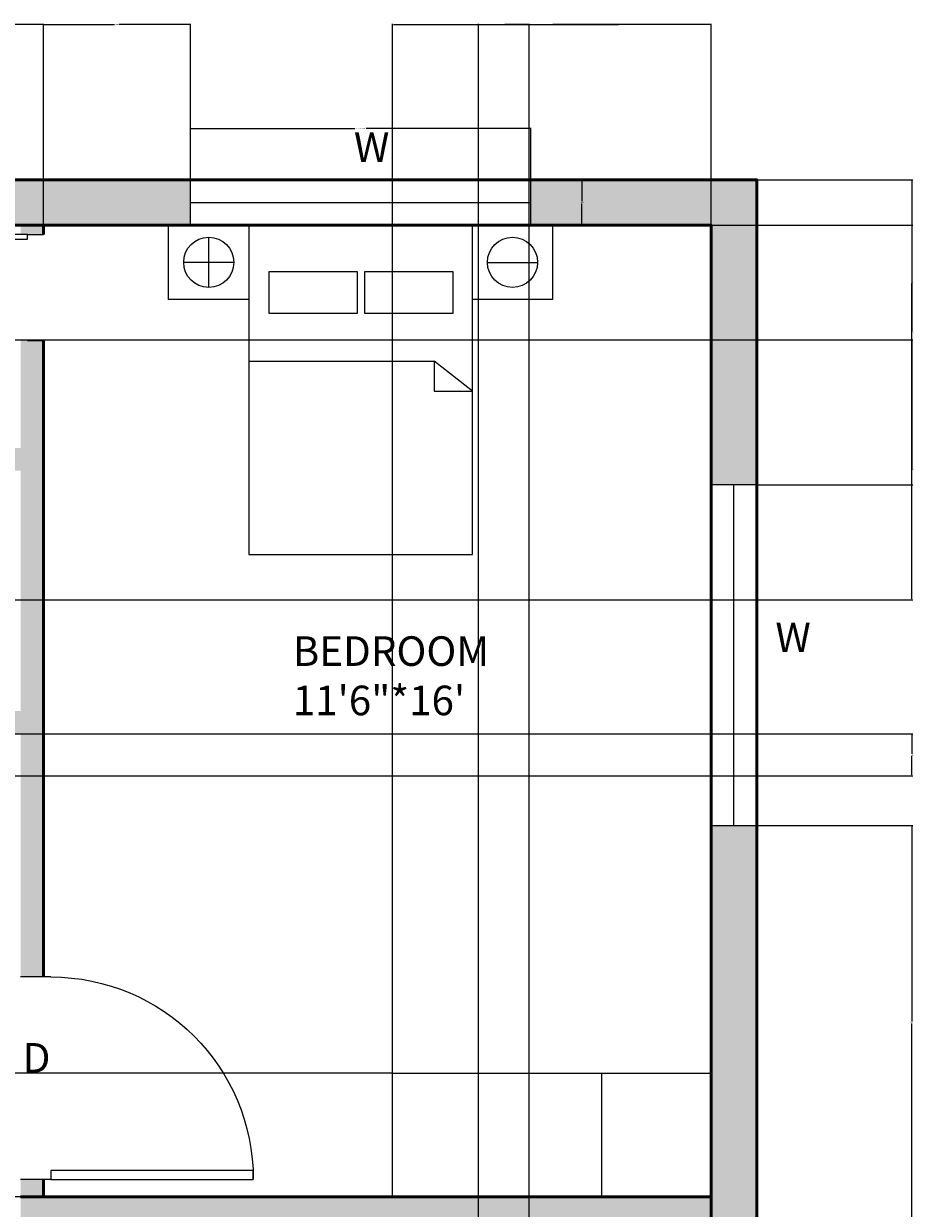
# Model space of a CAD drawing. Units: inches. Extents: x 678 to 1100, y 1432 to 2094.
# Tile 5 of 5: x 924 to 1100, y 1860 to 2094. Entities that reach past the tile are written whole.
import ezdxf

# ---------------------------------------------------------------- set-up
doc = ezdxf.new("R2010")
doc.units = ezdxf.units.IN
for name, color, linetype, lineweight in [('A-ANNO-DIMS', 2, 'Continuous', 18), ('A-AREA-IDEN', 141, 'Continuous', 25), ('A-FLOR-CASE', 30, 'Continuous', 25), ('A-WALL-PATT', 252, 'Continuous', 13), ('DOOR', 52, 'Continuous', 25), ('FUR', 30, 'Continuous', 18), ('TEXT', 141, 'Continuous', 18), ('WALL', 140, 'Continuous', 50), ('WIND', 212, 'Continuous', 25)]:
    doc.layers.add(name, color=color, linetype=linetype, lineweight=lineweight)
doc.styles.get("Standard").update_dxf_attribs({"font": 'arial.ttf'})
doc.dimstyles.get("Standard").update_dxf_attribs({"dimtxt": 0.18, "dimasz": 0.18, "dimexe": 0.18, "dimexo": 0.0625, "dimgap": 0.09, "dimtad": 0, "dimtih": 1, "dimtoh": 1, "dimdec": 4, "dimzin": 0, "dimdsep": 46, "dimtxsty": 'Standard', "dimcen": 0.09, "dimadec": 0, "dimazin": 0, "dimtfac": 1, "dimtdec": 4, "dimtofl": 0, "dimtmove": 0, "dimatfit": 3, "dimfxl": 1, "dimtolj": 1, "dimtzin": 0, "dimarcsym": 0})

# ---------------------------------------------------------------- blocks, each defined once
blk = doc.blocks.new('*U2')
for p, q in [((0, 0), (0, -6)), ((40, 0), (40, -6))]:
    blk.add_line(p, q)
blk.add_lwpolyline([(0, 0), (0, 40), (1.75, 40), (1.75, 0)], close=True)
blk.add_arc((0, 0), 40, 0, 90)
blk = doc.blocks.new('BED')
for p, q in [((0, 38.19), (36.64, 38.19)), ((36.64, 38.19), (36.64, 32.24)), ((44.21, 32.24), (36.64, 38.19)), ((36.64, 32.24), (44.21, 32.24))]:
    blk.add_line(p, q)
for points in [[(44.21, 65.05), (0, 65.05), (0, 0), (44.21, 0)], [(4.01, 55.91), (21.41, 55.91), (21.41, 47.59), (4.01, 47.59)], [(22.97, 55.91), (40.37, 55.91), (40.37, 47.59), (22.97, 47.59)]]:
    blk.add_lwpolyline(points, close=True)
blk = doc.blocks.new('NIGHTSTAND-LAMP')
for p, q in [((7.92, 2.38), (7.92, 12.28)), ((2.97, 7.33), (12.87, 7.33))]:
    blk.add_line(p, q)
blk.add_lwpolyline([(0, 14.65), (15.83, 14.65), (15.83, 0), (0, 0)], close=True)
blk.add_circle((7.92, 7.33), 4.95)
blk = doc.blocks.new('WIN-STANDARD')
blk.add_line((4.5, 0), (4.5, 67.31))
blk.add_lwpolyline([(9, 67.31), (0, 67.31), (0, 0), (9, 0)], close=True)
blk = doc.blocks.new('*D20')
at = {"layer": 'A-ANNO-DIMS', "color": 0, "lineweight": -2, "transparency": 16777216}
for p, q in [((957.01, 2062.99), (957.01, 2073.21)), ((957.19, 2073.03), (989.54, 2073.03)), ((1024.14, 2073.03), (991.78, 2073.03)), ((1024.32, 2062.99), (1024.32, 2073.21))]:
    blk.add_line(p, q, dxfattribs=at)
at = {"layer": 'A-ANNO-DIMS', "color": 0, "transparency": 16777216}
for points in [[(957.19, 2073.06), (957.19, 2073), (957.01, 2073.03)], [(1024.14, 2073.06), (1024.14, 2073), (1024.32, 2073.03)]]:
    blk.add_solid(points, dxfattribs=at)
at = {"layer": 'Defpoints', "color": 0, "transparency": 16777216}
for p in [(1024.32, 2073.03), (957.01, 2062.93), (1024.32, 2062.93)]:
    blk.add_point(p, dxfattribs=at)
at = {"layer": 'A-ANNO-DIMS', "color": 0, "transparency": 16777216, "insert": (990.66, 2073.03), "char_height": 0.18, "attachment_point": 5}
blk.add_mtext('\\A1;WINDOW 67 TYP.', dxfattribs=at)
blk = doc.blocks.new('*D21')
at = {"layer": 'A-ANNO-DIMS', "color": 0, "lineweight": -2, "transparency": 16777216}
for p, q in [((1024.38, 2062.93), (1034.6, 2062.93)), ((1034.42, 2062.75), (1034.42, 2058.61)), ((1034.42, 2054.11), (1034.42, 2058.25)), ((1024.38, 2053.93), (1034.6, 2053.93))]:
    blk.add_line(p, q, dxfattribs=at)
at = {"layer": 'A-ANNO-DIMS', "color": 0, "transparency": 16777216}
for points in [[(1034.39, 2062.75), (1034.45, 2062.75), (1034.42, 2062.93)], [(1034.39, 2054.11), (1034.45, 2054.11), (1034.42, 2053.93)]]:
    blk.add_solid(points, dxfattribs=at)
at = {"layer": 'Defpoints', "color": 0, "transparency": 16777216}
for p in [(1024.32, 2062.93), (1024.32, 2053.93), (1034.42, 2053.93)]:
    blk.add_point(p, dxfattribs=at)
at = {"layer": 'A-ANNO-DIMS', "color": 0, "transparency": 16777216, "insert": (1034.42, 2058.43), "char_height": 0.18, "attachment_point": 5}
blk.add_mtext('\\A1;9 TYP.', dxfattribs=at)
blk = doc.blocks.new('*D29')
at = {"layer": 'A-ANNO-DIMS', "color": 0, "lineweight": -2, "transparency": 16777216}
for p, q in [((896.07, 2062.99), (896.07, 2093.76)), ((896.25, 2093.58), (911.62, 2093.58)), ((927.78, 2093.58), (912.41, 2093.58)), ((927.96, 2053.99), (927.96, 2093.76))]:
    blk.add_line(p, q, dxfattribs=at)
at = {"layer": 'A-ANNO-DIMS', "color": 0, "transparency": 16777216}
for points in [[(896.25, 2093.61), (896.25, 2093.55), (896.07, 2093.58)], [(927.78, 2093.61), (927.78, 2093.55), (927.96, 2093.58)]]:
    blk.add_solid(points, dxfattribs=at)
at = {"layer": 'Defpoints', "color": 0, "transparency": 16777216}
for p in [(927.96, 2093.58), (896.07, 2062.93), (927.96, 2053.93)]:
    blk.add_point(p, dxfattribs=at)
at = {"layer": 'A-ANNO-DIMS', "color": 0, "transparency": 16777216, "insert": (912.02, 2093.58), "char_height": 0.18, "attachment_point": 5}
blk.add_mtext('\\A1;31.89', dxfattribs=at)
blk = doc.blocks.new('*D30')
at = {"layer": 'A-ANNO-DIMS', "color": 0, "lineweight": -2, "transparency": 16777216}
for p, q in [((927.96, 2053.99), (927.96, 2093.76)), ((928.14, 2093.58), (942.02, 2093.58)), ((956.83, 2093.58), (942.95, 2093.58)), ((957.01, 2062.99), (957.01, 2093.76))]:
    blk.add_line(p, q, dxfattribs=at)
at = {"layer": 'A-ANNO-DIMS', "color": 0, "transparency": 16777216}
for points in [[(928.14, 2093.61), (928.14, 2093.55), (927.96, 2093.58)], [(956.83, 2093.61), (956.83, 2093.55), (957.01, 2093.58)]]:
    blk.add_solid(points, dxfattribs=at)
at = {"layer": 'Defpoints', "color": 0, "transparency": 16777216}
for p in [(957.01, 2093.58), (957.01, 2062.93), (927.96, 2053.93)]:
    blk.add_point(p, dxfattribs=at)
at = {"layer": 'A-ANNO-DIMS', "color": 0, "transparency": 16777216, "insert": (942.48, 2093.58), "char_height": 0.18, "attachment_point": 5}
blk.add_mtext('\\A1;29.046', dxfattribs=at)
blk = doc.blocks.new('*D39')
at = {"layer": 'A-ANNO-DIMS', "color": 0, "lineweight": -2, "transparency": 16777216}
for p, q in [((1069.02, 1935.32), (1099.79, 1935.32)), ((1099.61, 1935.14), (1099.61, 1896.56)), ((1099.61, 1857.61), (1099.61, 1896.19)), ((1060.02, 1857.43), (1099.79, 1857.43))]:
    blk.add_line(p, q, dxfattribs=at)
at = {"layer": 'A-ANNO-DIMS', "color": 0, "transparency": 16777216}
for points in [[(1099.58, 1935.14), (1099.64, 1935.14), (1099.61, 1935.32)], [(1099.58, 1857.61), (1099.64, 1857.61), (1099.61, 1857.43)]]:
    blk.add_solid(points, dxfattribs=at)
at = {"layer": 'Defpoints', "color": 0, "transparency": 16777216}
for p in [(1068.96, 1935.32), (1099.61, 1935.32), (1059.96, 1857.43)]:
    blk.add_point(p, dxfattribs=at)
at = {"layer": 'A-ANNO-DIMS', "color": 0, "transparency": 16777216, "insert": (1099.61, 1896.38), "char_height": 0.18, "attachment_point": 5}
blk.add_mtext('\\A1;77.9', dxfattribs=at)
blk = doc.blocks.new('*D40')
at = {"layer": 'A-ANNO-DIMS', "color": 0, "lineweight": -2, "transparency": 16777216}
for p, q in [((1069.02, 2062.93), (1099.79, 2062.93)), ((1099.61, 2062.75), (1099.61, 2032.96)), ((1099.61, 2002.82), (1099.61, 2032.6)), ((1069.02, 2002.64), (1099.79, 2002.64))]:
    blk.add_line(p, q, dxfattribs=at)
at = {"layer": 'A-ANNO-DIMS', "color": 0, "transparency": 16777216}
for points in [[(1099.58, 2062.75), (1099.64, 2062.75), (1099.61, 2062.93)], [(1099.58, 2002.82), (1099.64, 2002.82), (1099.61, 2002.64)]]:
    blk.add_solid(points, dxfattribs=at)
at = {"layer": 'Defpoints', "color": 0, "transparency": 16777216}
for p in [(1068.96, 2062.93), (1099.61, 2062.93), (1068.96, 2002.64)]:
    blk.add_point(p, dxfattribs=at)
at = {"layer": 'A-ANNO-DIMS', "color": 0, "transparency": 16777216, "insert": (1099.61, 2032.78), "char_height": 0.18, "attachment_point": 5}
blk.add_mtext('\\A1;60.29', dxfattribs=at)
blk = doc.blocks.new('*D42')
at = {"layer": 'A-ANNO-DIMS', "color": 0, "lineweight": -2, "transparency": 16777216}
for p, q in [((718.02, 1953.43), (1099.79, 1953.43)), ((1099.61, 1953.25), (1099.61, 1949.47)), ((1099.61, 1945.33), (1099.61, 1949.11)), ((718.02, 1945.15), (1099.79, 1945.15))]:
    blk.add_line(p, q, dxfattribs=at)
at = {"layer": 'A-ANNO-DIMS', "color": 0, "transparency": 16777216}
for points in [[(1099.58, 1953.25), (1099.64, 1953.25), (1099.61, 1953.43)], [(1099.58, 1945.33), (1099.64, 1945.33), (1099.61, 1945.15)]]:
    blk.add_solid(points, dxfattribs=at)
at = {"layer": 'Defpoints', "color": 0, "transparency": 16777216}
for p in [(717.96, 1953.43), (1099.61, 1953.43), (717.96, 1945.15)]:
    blk.add_point(p, dxfattribs=at)
at = {"layer": 'A-ANNO-DIMS', "color": 0, "transparency": 16777216, "insert": (1099.61, 1949.29), "char_height": 0.18, "attachment_point": 5}
blk.add_mtext('\\A1;8.282', dxfattribs=at)
blk = doc.blocks.new('*D43')
at = {"layer": 'A-ANNO-DIMS', "color": 0, "lineweight": -2, "transparency": 16777216}
for p, q in [((718.02, 2031.32), (1099.79, 2031.32)), ((1099.61, 2031.14), (1099.61, 2005.81)), ((1099.61, 1980.12), (1099.61, 2005.45)), ((718.02, 1979.94), (1099.79, 1979.94))]:
    blk.add_line(p, q, dxfattribs=at)
at = {"layer": 'A-ANNO-DIMS', "color": 0, "transparency": 16777216}
for points in [[(1099.58, 2031.14), (1099.64, 2031.14), (1099.61, 2031.32)], [(1099.58, 1980.12), (1099.64, 1980.12), (1099.61, 1979.94)]]:
    blk.add_solid(points, dxfattribs=at)
at = {"layer": 'Defpoints', "color": 0, "transparency": 16777216}
for p in [(717.96, 2031.32), (1099.61, 2031.32), (717.96, 1979.94)]:
    blk.add_point(p, dxfattribs=at)
at = {"layer": 'A-ANNO-DIMS', "color": 0, "transparency": 16777216, "insert": (1099.61, 2005.63), "char_height": 0.18, "attachment_point": 5}
blk.add_mtext('\\A1;51.38', dxfattribs=at)
blk = doc.blocks.new('*D44')
at = {"layer": 'A-ANNO-DIMS', "color": 0, "lineweight": -2, "transparency": 16777216}
for p, q in [((718.02, 2053.93), (1099.79, 2053.93)), ((1099.61, 2053.75), (1099.61, 2042.81)), ((1099.61, 2031.5), (1099.61, 2042.44)), ((718.02, 2031.32), (1099.79, 2031.32))]:
    blk.add_line(p, q, dxfattribs=at)
at = {"layer": 'A-ANNO-DIMS', "color": 0, "transparency": 16777216}
for points in [[(1099.58, 2053.75), (1099.64, 2053.75), (1099.61, 2053.93)], [(1099.58, 2031.5), (1099.64, 2031.5), (1099.61, 2031.32)]]:
    blk.add_solid(points, dxfattribs=at)
at = {"layer": 'Defpoints', "color": 0, "transparency": 16777216}
for p in [(717.96, 2053.93), (1099.61, 2053.93), (717.96, 2031.32)]:
    blk.add_point(p, dxfattribs=at)
at = {"layer": 'A-ANNO-DIMS', "color": 0, "transparency": 16777216, "insert": (1099.61, 2042.62), "char_height": 0.18, "attachment_point": 5}
blk.add_mtext('\\A1;22.61', dxfattribs=at)
blk = doc.blocks.new('*D49')
at = {"layer": 'A-ANNO-DIMS', "color": 0, "lineweight": -2, "transparency": 16777216}
for p, q in [((1013.96, 1471.99), (1013.96, 2093.76)), ((1014.14, 2093.58), (1018.75, 2093.58)), ((1023.78, 2093.58), (1019.17, 2093.58)), ((1023.96, 1471.99), (1023.96, 2093.76))]:
    blk.add_line(p, q, dxfattribs=at)
at = {"layer": 'A-ANNO-DIMS', "color": 0, "transparency": 16777216}
for points in [[(1014.14, 2093.61), (1014.14, 2093.55), (1013.96, 2093.58)], [(1023.78, 2093.61), (1023.78, 2093.55), (1023.96, 2093.58)]]:
    blk.add_solid(points, dxfattribs=at)
at = {"layer": 'Defpoints', "color": 0, "transparency": 16777216}
for p in [(1023.96, 2093.58), (1013.96, 1471.93), (1023.96, 1471.93)]:
    blk.add_point(p, dxfattribs=at)
at = {"layer": 'A-ANNO-DIMS', "color": 0, "transparency": 16777216, "insert": (1018.96, 2093.58), "char_height": 0.18, "attachment_point": 5}
blk.add_mtext('\\A1;10', dxfattribs=at)
blk = doc.blocks.new('*D50')
at = {"layer": 'A-ANNO-DIMS', "color": 0, "lineweight": -2, "transparency": 16777216}
for p, q in [((1023.96, 1471.99), (1023.96, 2093.76)), ((1024.14, 2093.58), (1041.74, 2093.58)), ((1059.78, 2093.58), (1042.18, 2093.58)), ((1059.96, 1471.99), (1059.96, 2093.76))]:
    blk.add_line(p, q, dxfattribs=at)
at = {"layer": 'A-ANNO-DIMS', "color": 0, "transparency": 16777216}
for points in [[(1024.14, 2093.61), (1024.14, 2093.55), (1023.96, 2093.58)], [(1059.78, 2093.61), (1059.78, 2093.55), (1059.96, 2093.58)]]:
    blk.add_solid(points, dxfattribs=at)
at = {"layer": 'Defpoints', "color": 0, "transparency": 16777216}
for p in [(1059.96, 2093.58), (1023.96, 1471.93), (1059.96, 1471.93)]:
    blk.add_point(p, dxfattribs=at)
at = {"layer": 'A-ANNO-DIMS', "color": 0, "transparency": 16777216, "insert": (1041.96, 2093.58), "char_height": 0.18, "attachment_point": 5}
blk.add_mtext('\\A1;36', dxfattribs=at)
blk = doc.blocks.new('*D57')
at = {"layer": 'A-ANNO-DIMS', "color": 0, "lineweight": -2, "transparency": 16777216}
for p, q in [((996.96, 1886.44), (996.96, 2093.76)), ((997.14, 2093.58), (1028.24, 2093.58)), ((1059.78, 2093.58), (1028.68, 2093.58)), ((1059.96, 1886.44), (1059.96, 2093.76))]:
    blk.add_line(p, q, dxfattribs=at)
at = {"layer": 'A-ANNO-DIMS', "color": 0, "transparency": 16777216}
for points in [[(997.14, 2093.61), (997.14, 2093.55), (996.96, 2093.58)], [(1059.78, 2093.61), (1059.78, 2093.55), (1059.96, 2093.58)]]:
    blk.add_solid(points, dxfattribs=at)
at = {"layer": 'Defpoints', "color": 0, "transparency": 16777216}
for p in [(1059.96, 2093.58), (996.96, 1886.38), (1059.96, 1886.38)]:
    blk.add_point(p, dxfattribs=at)
at = {"layer": 'A-ANNO-DIMS', "color": 0, "transparency": 16777216, "insert": (1028.46, 2093.58), "char_height": 0.18, "attachment_point": 5}
blk.add_mtext('\\A1;63', dxfattribs=at)
blk = doc.blocks.new('*D58')
at = {"layer": 'A-ANNO-DIMS', "color": 0, "lineweight": -2, "transparency": 16777216}
for p, q in [((996.9, 1886.38), (678.13, 1886.38)), ((678.31, 1886.2), (678.31, 1874.34)), ((678.31, 1862.11), (678.31, 1873.97)), ((996.9, 1861.93), (678.13, 1861.93))]:
    blk.add_line(p, q, dxfattribs=at)
at = {"layer": 'A-ANNO-DIMS', "color": 0, "transparency": 16777216}
for points in [[(678.28, 1886.2), (678.34, 1886.2), (678.31, 1886.38)], [(678.28, 1862.11), (678.34, 1862.11), (678.31, 1861.93)]]:
    blk.add_solid(points, dxfattribs=at)
at = {"layer": 'Defpoints', "color": 0, "transparency": 16777216}
for p in [(678.31, 1886.38), (996.96, 1886.38), (996.96, 1861.93)]:
    blk.add_point(p, dxfattribs=at)
at = {"layer": 'A-ANNO-DIMS', "color": 0, "transparency": 16777216, "insert": (678.31, 1874.15), "char_height": 0.18, "attachment_point": 5}
blk.add_mtext('\\A1;24.45', dxfattribs=at)

msp = doc.modelspace()

# ---------------------------------------------------------------- hatches: boundary and pattern name
at = {"layer": 'A-WALL-PATT'}
h = msp.add_hatch(color=256, dxfattribs=at)
h.dxf.hatch_style = 1
h.paths.add_polyline_path([(859.7133, 2062.9286), (708.9606, 2062.9286), (708.9606, 2031.3203), (717.9606, 2031.3203), (717.9606, 2053.9286), (837.9606, 2053.9286), (859.7133, 2053.9286)])
h.paths.add_polyline_path([(957.0069, 2062.9286), (896.0724, 2062.9286), (896.0724, 2053.9286), (957.0069, 2053.9286)])
h.paths.add_polyline_path([(842.4606, 2053.9286), (837.9606, 2053.9286), (837.9606, 2005.4286), (842.4606, 2005.4286), (923.4606, 2005.4286), (923.4606, 2009.9286), (842.4606, 2009.9286)])
h.paths.add_polyline_path([(927.9606, 2053.9286), (923.4606, 2053.9286), (923.4606, 2052.1286), (924.8103, 2052.1286), (927.9606, 2052.1286)])
h.paths.add_polyline_path([(1068.9606, 2062.9286), (1024.3184, 2062.9286), (1024.3184, 2053.9286), (1028.6041, 2053.9286), (1059.9606, 2053.9286), (1059.9606, 2002.6361), (1068.9606, 2002.6361)])
h.paths.add_polyline_path([(1059.9606, 1861.9286), (996.9604, 1861.9286), (927.9606, 1861.9286), (923.4606, 1861.9286), (923.4606, 1857.4286), (1059.9606, 1857.4286)], flags=17)
h.paths.add_polyline_path([(927.9606, 2031.1269), (924.8103, 2031.1269, -0.01607952), (923.4606, 2031.1703), (923.4606, 1905.3856), (927.9606, 1905.3856)])
h.paths.add_polyline_path([(923.4606, 1957.9286), (842.4606, 1957.9286), (842.4606, 1969.339), (837.9606, 1969.339), (837.9606, 1953.4286), (923.4606, 1953.4286)])
h.paths.add_polyline_path([(774.6357, 1957.9286), (717.9606, 1957.9286), (717.9606, 1953.4286), (774.6357, 1953.4286)])
h.paths.add_polyline_path([(717.9606, 1979.9404), (708.9606, 1979.9404), (708.9606, 1945.1463), (717.9606, 1945.1463)])
h.paths.add_polyline_path([(840.5596, 1861.9286), (717.9606, 1861.9286), (717.9606, 1857.4286), (840.5596, 1857.4286)], flags=17)
h.paths.add_polyline_path([(927.9606, 1865.3856), (923.4606, 1865.3856), (923.4606, 1861.9286), (927.9606, 1861.9286)], flags=17)
h.paths.add_polyline_path([(1059.9606, 1689.4286), (967.3461, 1689.4286), (967.3461, 1684.9286), (1059.9606, 1684.9286)], flags=17)
h.paths.add_polyline_path([(987.9606, 1737.4286), (983.4606, 1737.4286), (983.4606, 1715.196), (986.7357, 1715.196, -0.01403382), (987.9606, 1715.1616)], flags=17)
h.paths.add_polyline_path([(916.0499, 2036.8414), (924.8721, 2036.8414), (924.8721, 2048.8901), (916.0499, 2048.8901)], flags=9)
h.paths.add_polyline_path([(921.7778, 1883.2914), (930.5999, 1883.2914), (930.5999, 1895.3401), (921.7778, 1895.3401)], flags=25)
h.paths.add_polyline_path([(732.1085, 1683.0506), (740.9307, 1683.0506), (740.9307, 1695.0993), (732.1085, 1695.0993)], flags=25)
h.paths.add_polyline_path([(943.8458, 1737.5114), (952.6679, 1737.5114), (952.6679, 1749.5601), (943.8458, 1749.5601)], flags=25)
h.paths.add_polyline_path([(986.0751, 1696.9795), (994.8973, 1696.9795), (994.8973, 1709.0282), (986.0751, 1709.0282)], flags=25)
h.paths.add_polyline_path([(940.1881, 1677.378), (949.0103, 1677.378), (949.0103, 1689.4267), (940.1881, 1689.4267)], flags=25)
h.paths.add_polyline_path([(998.6262, 1761.7469), (1044.0453, 1761.7469), (1044.0453, 1783.5644), (998.6262, 1783.5644)], flags=25)
h.paths.add_polyline_path([(997.3001, 1713.4735), (1028.9316, 1713.4735), (1028.9316, 1735.2909), (997.3001, 1735.2909)], flags=25)
h.paths.add_polyline_path([(1005.9896, 1586.8139), (1051.4087, 1586.8139), (1051.4087, 1608.6313), (1005.9896, 1608.6313)], flags=25)
h.paths.add_polyline_path([(794.7038, 1552.8124), (873.8721, 1552.8124), (873.8721, 1574.6298), (794.7038, 1574.6298)], flags=25)
h.paths.add_polyline_path([(774.2693, 1771.1228), (831.9444, 1771.1228), (831.9444, 1792.9403), (774.2693, 1792.9403)], flags=25)
h.paths.add_polyline_path([(750.0357, 1897.1514), (786.4291, 1897.1514), (786.4291, 1918.9689), (750.0357, 1918.9689)], flags=25)
h.paths.add_polyline_path([(974.9086, 1953.7921), (1020.3276, 1953.7921), (1020.3276, 1975.6096), (974.9086, 1975.6096)], flags=9)
h.paths.add_polyline_path([(859.1564, 1973.8092), (890.2175, 1973.8092), (890.2175, 1995.6267), (859.1564, 1995.6267)], flags=9)
h.paths.add_polyline_path([(753.2305, 1989.0219), (792.2962, 1989.0219), (792.2962, 2010.8393), (753.2305, 2010.8393)], flags=9)
h.paths.add_polyline_path([(1067.3992, 1620.1515), (1078.032, 1620.1515), (1078.032, 1632.2002), (1067.3992, 1632.2002)], flags=9)
h.paths.add_polyline_path([(846.8446, 2028.8178), (878.5079, 2028.8178), (878.5079, 2050.6353), (846.8446, 2050.6353)], flags=25)
h.paths.add_polyline_path([(1059.9606, 1832.7202), (1068.9606, 1832.7202), (1068.9606, 1935.3246), (1059.9606, 1935.3246)])
h.paths.add_polyline_path([(1068.9606, 1765.4088), (1059.9606, 1765.4088), (1059.9606, 1728.1446), (1068.9606, 1728.1446)])
h.paths.add_polyline_path([(1059.9606, 1657.7018), (1068.9606, 1657.7018), (1068.9606, 1697.8017), (1059.9606, 1697.8017)])
h.paths.add_polyline_path([(1068.9606, 1590.3903), (1059.9606, 1590.3903), (1059.9606, 1551.1623), (1068.9606, 1551.1623)])
h.paths.add_polyline_path([(708.9606, 1826.8331), (717.9606, 1826.8331), (717.9606, 1877.8348), (708.9606, 1877.8348)])
h.paths.add_polyline_path([(717.9606, 1759.5217), (708.9606, 1759.5217), (708.9606, 1462.9286), (1068.9606, 1462.9286), (1068.9606, 1483.8508), (1059.9606, 1483.8508), (1059.9606, 1471.9286), (717.9606, 1471.9286)])
h = msp.add_hatch(color=256, dxfattribs=at)
h.dxf.hatch_style = 1
h.paths.add_polyline_path([(1059.9606, 1741.9286), (970.7942, 1741.9286), (970.7942, 1737.4286), (1059.9606, 1737.4286)])
h.paths.add_polyline_path([(927.3461, 1689.4286), (759.4099, 1689.4286), (759.4099, 1684.9286), (927.3461, 1684.9286)])
h.paths.add_polyline_path([(921.9606, 1684.9286), (917.4606, 1684.9286), (917.4606, 1560.4286), (921.9606, 1560.4286)])
h.paths.add_polyline_path([(1059.9606, 1564.9286), (921.9606, 1564.9286), (921.9606, 1560.4286), (1059.9606, 1560.4286)])
h.paths.add_polyline_path([(916.0499, 2036.8414), (924.8721, 2036.8414), (924.8721, 2048.8901), (916.0499, 2048.8901)], flags=9)
h.paths.add_polyline_path([(921.7778, 1883.2914), (930.5999, 1883.2914), (930.5999, 1895.3401), (921.7778, 1895.3401)], flags=9)
h.paths.add_polyline_path([(732.1085, 1683.0506), (740.9307, 1683.0506), (740.9307, 1695.0993), (732.1085, 1695.0993)], flags=9)
h.paths.add_polyline_path([(943.8458, 1737.5114), (952.6679, 1737.5114), (952.6679, 1749.5601), (943.8458, 1749.5601)], flags=9)
h.paths.add_polyline_path([(986.0751, 1696.9795), (994.8973, 1696.9795), (994.8973, 1709.0282), (986.0751, 1709.0282)], flags=9)
h.paths.add_polyline_path([(940.1881, 1677.378), (949.0103, 1677.378), (949.0103, 1689.4267), (940.1881, 1689.4267)], flags=9)
h.paths.add_polyline_path([(998.6262, 1761.7469), (1044.0453, 1761.7469), (1044.0453, 1783.5644), (998.6262, 1783.5644)], flags=9)
h.paths.add_polyline_path([(1005.9896, 1586.8139), (1051.4087, 1586.8139), (1051.4087, 1608.6313), (1005.9896, 1608.6313)], flags=9)
h.paths.add_polyline_path([(794.7038, 1552.8124), (873.8721, 1552.8124), (873.8721, 1574.6298), (794.7038, 1574.6298)], flags=9)
h.paths.add_polyline_path([(774.2693, 1771.1228), (831.9444, 1771.1228), (831.9444, 1792.9403), (774.2693, 1792.9403)], flags=9)
h.paths.add_polyline_path([(750.0357, 1897.1514), (786.4291, 1897.1514), (786.4291, 1918.9689), (750.0357, 1918.9689)], flags=9)
h.paths.add_polyline_path([(974.9086, 1953.7921), (1020.3276, 1953.7921), (1020.3276, 1975.6096), (974.9086, 1975.6096)], flags=9)
h.paths.add_polyline_path([(859.1564, 1973.8092), (890.2175, 1973.8092), (890.2175, 1995.6267), (859.1564, 1995.6267)], flags=9)
h.paths.add_polyline_path([(846.8446, 2028.8178), (878.5079, 2028.8178), (878.5079, 2050.6353), (846.8446, 2050.6353)], flags=9)
h.paths.add_polyline_path([(753.2305, 1989.0219), (792.2962, 1989.0219), (792.2962, 2010.8393), (753.2305, 2010.8393)], flags=9)
h = msp.add_hatch(color=256, dxfattribs=at)
h.dxf.hatch_style = 1
h.paths.add_polyline_path([(927.9606, 1857.4286), (923.4606, 1857.4286), (923.4606, 1737.4286), (927.9606, 1737.4286)])
h.paths.add_polyline_path([(930.7942, 1741.9286), (927.9606, 1741.9286), (927.9606, 1737.4286), (930.7942, 1737.4286)])
h.paths.add_polyline_path([(916.0499, 2036.8414), (924.8721, 2036.8414), (924.8721, 2048.8901), (916.0499, 2048.8901)], flags=9)
h.paths.add_polyline_path([(921.7778, 1883.2914), (930.5999, 1883.2914), (930.5999, 1895.3401), (921.7778, 1895.3401)], flags=9)
h.paths.add_polyline_path([(732.1085, 1683.0506), (740.9307, 1683.0506), (740.9307, 1695.0993), (732.1085, 1695.0993)], flags=9)
h.paths.add_polyline_path([(943.8458, 1737.5114), (952.6679, 1737.5114), (952.6679, 1749.5601), (943.8458, 1749.5601)], flags=9)
h.paths.add_polyline_path([(986.0751, 1696.9795), (994.8973, 1696.9795), (994.8973, 1709.0282), (986.0751, 1709.0282)], flags=9)
h.paths.add_polyline_path([(940.1881, 1677.378), (949.0103, 1677.378), (949.0103, 1689.4267), (940.1881, 1689.4267)], flags=9)
h.paths.add_polyline_path([(998.6262, 1761.7469), (1044.0453, 1761.7469), (1044.0453, 1783.5644), (998.6262, 1783.5644)], flags=9)
h.paths.add_polyline_path([(997.3001, 1713.4735), (1028.9316, 1713.4735), (1028.9316, 1735.2909), (997.3001, 1735.2909)], flags=9)
h.paths.add_polyline_path([(1005.9896, 1586.8139), (1051.4087, 1586.8139), (1051.4087, 1608.6313), (1005.9896, 1608.6313)], flags=9)
h.paths.add_polyline_path([(794.7038, 1552.8124), (873.8721, 1552.8124), (873.8721, 1574.6298), (794.7038, 1574.6298)], flags=9)
h.paths.add_polyline_path([(774.2693, 1771.1228), (831.9444, 1771.1228), (831.9444, 1792.9403), (774.2693, 1792.9403)], flags=9)
h.paths.add_polyline_path([(750.0357, 1897.1514), (786.4291, 1897.1514), (786.4291, 1918.9689), (750.0357, 1918.9689)], flags=9)
h.paths.add_polyline_path([(974.9086, 1953.7921), (1020.3276, 1953.7921), (1020.3276, 1975.6096), (974.9086, 1975.6096)], flags=9)
h.paths.add_polyline_path([(859.1564, 1973.8092), (890.2175, 1973.8092), (890.2175, 1995.6267), (859.1564, 1995.6267)], flags=9)
h.paths.add_polyline_path([(846.8446, 2028.8178), (878.5079, 2028.8178), (878.5079, 2050.6353), (846.8446, 2050.6353)], flags=9)
h.paths.add_polyline_path([(753.2305, 1989.0219), (792.2962, 1989.0219), (792.2962, 2010.8393), (753.2305, 2010.8393)], flags=9)

# ---------------------------------------------------------------- linework, layer by layer
at = {"layer": 'A-FLOR-CASE'}
msp.add_line((1038.3562, 1861.9286), (1038.3562, 1886.3805), dxfattribs=at)
msp.add_lwpolyline([(1059.9606, 1861.9286), (996.9604, 1861.9286), (996.9604, 1886.3805), (1059.9606, 1886.3805)], close=True, dxfattribs=at)
at = {"layer": 'FUR'}
msp.add_line((1015.7347, 2046.6015), (1025.6387, 2046.6015), dxfattribs=at)
msp.add_lwpolyline([(1012.7693, 2053.9286), (1028.6041, 2053.9286), (1028.6041, 2039.2744), (1012.7693, 2039.2744)], close=True, dxfattribs=at)
msp.add_circle((1020.6867, 2046.6015), 4.952, dxfattribs=at)
at = {"layer": 'WALL'}
for p, q in [((708.9606, 2062.9286), (1068.9606, 2062.9286)), ((1068.9606, 2062.9286), (1068.9606, 1462.9286)), ((1059.9606, 2053.9286), (927.9606, 2053.9286)), ((927.9606, 2053.9286), (927.9606, 2052.1286)), ((927.9606, 2031.1269), (927.9606, 1905.3856)), ((927.9606, 1865.3856), (927.9606, 1861.9286)), ((927.9606, 1861.9286), (923.4606, 1861.9286)), ((927.9606, 1861.9286), (1059.9606, 1861.9286))]:
    msp.add_line(p, q, dxfattribs=at)
for points in [[(708.9606, 2062.9286), (1068.9606, 2062.9286), (1068.9606, 1462.9286), (708.9606, 1462.9286)], [(717.9606, 2053.9286), (1059.9606, 2053.9286), (1059.9606, 1471.9286), (717.9606, 1471.9286)]]:
    msp.add_lwpolyline(points, close=True, dxfattribs=at)

# ---------------------------------------------------------------- block references
at = {"layer": 'DOOR', "xscale": -0.5250429133739555, "yscale": 0.5250429133739555, "zscale": 0.5250429133739555, "rotation": 90}
msp.add_blockref('*U2', (924.8103, 2052.1286), dxfattribs=at)
at = {"layer": 'DOOR', "xscale": -1, "rotation": 270}
msp.add_blockref('*U2', (929.4606, 1865.3856), dxfattribs=at)
at = {"layer": 'FUR'}
for name, p in [('NIGHTSTAND-LAMP', (952.7215, 2039.274)), ('BED', (968.5556, 1988.879))]:
    msp.add_blockref(name, p, dxfattribs=at)
at = {"layer": 'WIND', "rotation": 269.9999999999991}
msp.add_blockref('WIN-STANDARD', (957.0071, 2062.9282), dxfattribs=at)
at = {"layer": 'WIND'}
msp.add_blockref('WIN-STANDARD', (1059.961, 1935.3248), dxfattribs=at)

# ---------------------------------------------------------------- texts
at = {"layer": 'A-AREA-IDEN', "insert": (977.2597, 1972.7041), "char_height": 5.84689, "attachment_point": 1}
msp.add_mtext_dynamic_manual_height_columns('BEDROOM\\P11\'6"*16\'', width=180.890738, gutter_width=29.2344, heights=[0], dxfattribs=at)
at = {"layer": 'TEXT', "char_height": 5.8469, "attachment_point": 1}
for s, insert in [('W', (989.3459, 2072.277)), ('W', (1072.6487, 1975.4259)), ('D', (923.8696, 1892.331))]:
    msp.add_mtext_dynamic_manual_height_columns(s, width=180.890738, gutter_width=29.2344, heights=[0], dxfattribs=dict(at, insert=insert))

# ---------------------------------------------------------------- dimensions: what is measured, and where the dimension line sits
at = {"layer": 'A-ANNO-DIMS'}
for base, p1, p2, override, picture, middle in [((927.9606, 2093.5786), (896.0724, 2062.9286), (927.9606, 2053.9286), {"dimdec": 2, "dimlfac": 1, "dimrnd": 0, "dimzin": 0, "dimdsep": 46, "dimlunit": 2}, '*D29', (912.0165, 2093.5786)), ((957.0069, 2093.5786), (927.9606, 2053.9286), (957.0069, 2062.9286), {"dimdec": 3, "dimlfac": 1, "dimrnd": 0, "dimzin": 0, "dimdsep": 46, "dimlunit": 2}, '*D30', (942.4838, 2093.5786)), ((1059.9606, 2093.5786), (996.9604, 1886.3805), (1059.9606, 1886.3805), {"dimdec": 0, "dimlfac": 1, "dimrnd": 0, "dimzin": 0, "dimdsep": 46, "dimlunit": 2}, '*D57', (1028.4605, 2093.5786)), ((1023.9606, 2093.5786), (1013.9606, 1471.9286), (1023.9606, 1471.9286), {"dimdec": 0, "dimlfac": 1, "dimrnd": 0, "dimzin": 0, "dimdsep": 46, "dimlunit": 2}, '*D49', (1018.9606, 2093.5786)), ((1059.9606, 2093.5786), (1023.9606, 1471.9286), (1059.9606, 1471.9286), {"dimdec": 0, "dimlfac": 1, "dimrnd": 0, "dimzin": 0, "dimdsep": 46, "dimlunit": 2}, '*D50', (1041.9606, 2093.5786))]:
    dim = msp.add_linear_dim(base=base, p1=p1, p2=p2, dimstyle='Standard', override=override, dxfattribs=at)
    dim.commit()
    dim.dimension.update_dxf_attribs({"geometry": picture, "text_midpoint": middle})
dim = msp.add_linear_dim(base=(1024.3184, 2073.0253), p1=(957.0069, 2062.9286), p2=(1024.3184, 2062.9286), text='WINDOW <> TYP.', dimstyle='Standard', override={"dimdec": 0, "dimlfac": 1, "dimrnd": 0, "dimzin": 0, "dimdsep": 46, "dimlunit": 2}, dxfattribs=at)
dim.commit()
dim.dimension.update_dxf_attribs({"geometry": '*D20', "text_midpoint": (990.6626, 2073.0253)})
dim = msp.add_linear_dim(base=(1034.4151, 2053.9286), p1=(1024.3184, 2062.9286), p2=(1024.3184, 2053.9286), angle=270, text='<> TYP.', dimstyle='Standard', override={"dimdec": 0, "dimlfac": 1, "dimrnd": 0, "dimzin": 0, "dimdsep": 46, "dimlunit": 2}, dxfattribs=at)
dim.commit()
dim.dimension.update_dxf_attribs({"geometry": '*D21', "text_midpoint": (1034.4151, 2058.4286)})
for base, p1, p2, override, picture, middle in [((1099.6106, 2062.9286), (1068.9606, 2002.6361), (1068.9606, 2062.9286), {"dimdec": 2, "dimlfac": 1, "dimrnd": 0, "dimzin": 0, "dimdsep": 46, "dimlunit": 2}, '*D40', (1099.6106, 2032.7823)), ((1099.6106, 2053.9286), (717.9606, 2031.3203), (717.9606, 2053.9286), {"dimdec": 2, "dimlfac": 1, "dimrnd": 0, "dimzin": 0, "dimdsep": 46, "dimlunit": 2}, '*D44', (1099.6106, 2042.6244)), ((1099.6106, 2031.3203), (717.9606, 1979.9404), (717.9606, 2031.3203), {"dimdec": 2, "dimlfac": 1, "dimrnd": 0, "dimzin": 0, "dimdsep": 46, "dimlunit": 2}, '*D43', (1099.6106, 2005.6303)), ((1099.6106, 1953.4286), (717.9606, 1945.1463), (717.9606, 1953.4286), {"dimdec": 3, "dimlfac": 1, "dimrnd": 0, "dimzin": 0, "dimdsep": 46, "dimlunit": 2}, '*D42', (1099.6106, 1949.2874)), ((1099.6106, 1935.3246), (1059.9606, 1857.4286), (1068.9606, 1935.3246), {"dimdec": 1, "dimlfac": 1, "dimrnd": 0, "dimzin": 0, "dimdsep": 46, "dimlunit": 2}, '*D39', (1099.6106, 1896.3766)), ((678.3106, 1886.3805), (996.9604, 1861.9286), (996.9604, 1886.3805), {"dimdec": 2, "dimlfac": 1, "dimrnd": 0, "dimzin": 0, "dimdsep": 46, "dimlunit": 2}, '*D58', (678.3106, 1874.1545))]:
    dim = msp.add_linear_dim(base=base, p1=p1, p2=p2, angle=90, dimstyle='Standard', override=override, dxfattribs=at)
    dim.commit()
    dim.dimension.update_dxf_attribs({"geometry": picture, "text_midpoint": middle})

doc.saveas('drawing.dxf')
